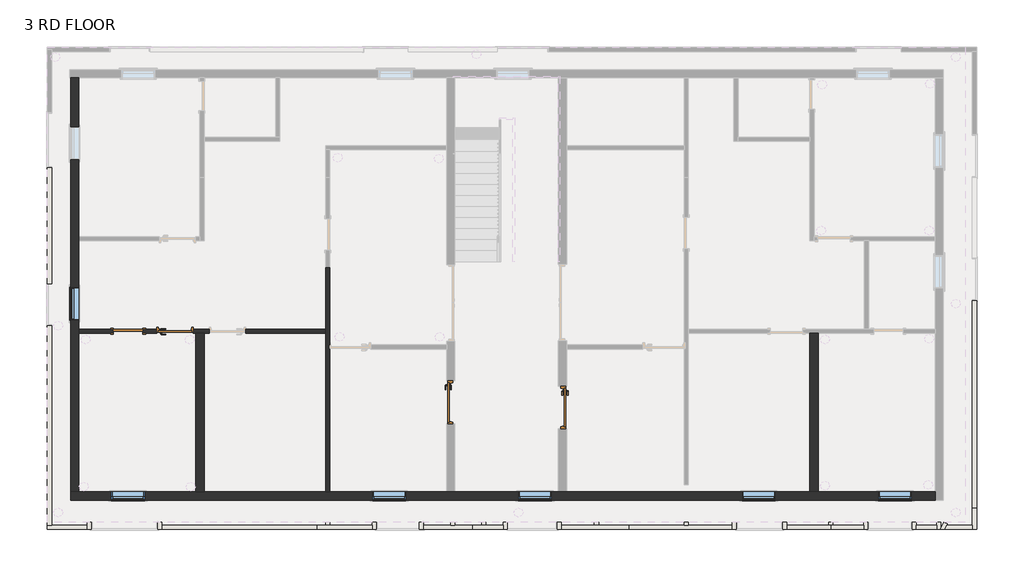
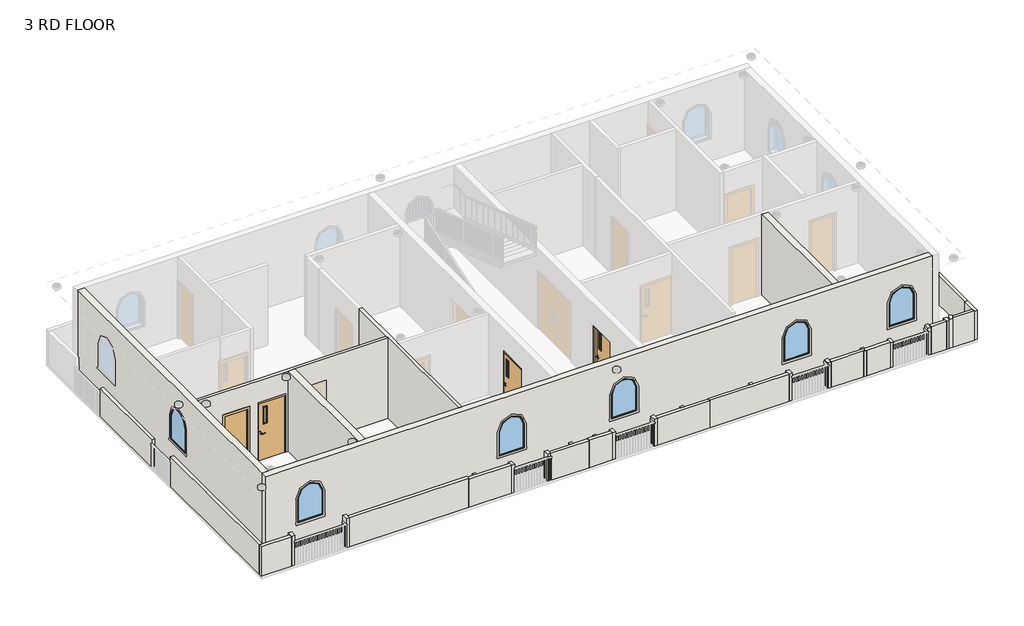
# One storey, part 1 of 7: 39 walls, 6 windows, 4 doors.
# Revit data of these elements (continued)
# Element 4 (IfcDoor, "Single-Flush : 2'8\"x 7'") (continued)
#   Phase Created = New Construction
#   Materials on its faces: "Door - Frame", "Door - Panel"
# Elements 5, 6 (IfcWall, "Generic - 4.5\"")
#   Top Offset = -0' - 6"
#   Base Offset = 0' - 0"
#   wall height = 10' - 0"
#   Phase Created = New Construction
#   Base Constraint = 3 RD FLOOR
#   Top Constraint = 4 TH FLOOR
#   Materials on its faces: "Default Wall"
# Element 7 (IfcWall, "Generic - 4.5\"")
#   Top Offset = -6' - 10.1834"
#   Base Offset = 0' - 0"
#   wall height = 3' - 7.8166"
#   Phase Created = New Construction
#   Base Constraint = 3 RD FLOOR
#   Top Constraint = 4 TH FLOOR
#   Materials on its faces: "Default Wall"
# Element 8 (IfcWall, "Generic - 4.5\"")
#   Top Offset = 0' - 0"
#   Base Offset = 0' - 0"
#   Unconnected Height = 3' - 8.64293"
#   wall height = 3' - 8.64293"
#   Phase Created = New Construction
#   Base Constraint = 3 RD FLOOR
#   Materials on its faces: "Default Wall"
# Element 9 (IfcWall, "Generic - 4.5\"")
#   Top Offset = -6' - 10.57009"
#   Base Offset = 0' - 0"
#   wall height = 3' - 7.42991"
#   Phase Created = New Construction
#   Base Constraint = 3 RD FLOOR
#   Top Constraint = 4 TH FLOOR
#   Materials on its faces: "Default Wall"
# Element 10 (IfcWall, "Generic - 4.5\"")
#   Top Offset = -6' - 11.10495"
#   Base Offset = 0' - 0"
#   wall height = 3' - 6.89505"
#   Phase Created = New Construction
#   Base Constraint = 3 RD FLOOR
#   Top Constraint = 4 TH FLOOR
#   Materials on its faces: "Default Wall"
# Element 11 (IfcWall, "Generic - 4.5\"")
#   Top Offset = -6' - 11.01332"
#   Base Offset = 0' - 0"
#   wall height = 3' - 6.98668"
#   Phase Created = New Construction
#   Base Constraint = 3 RD FLOOR
#   Top Constraint = 4 TH FLOOR
#   Materials on its faces: "Default Wall"
# Element 12 (IfcWall, "Generic - 4.5\"")
#   Top Offset = -7' - 0.14651"
#   Base Offset = 0' - 0"
#   wall height = 3' - 5.85349"
#   Phase Created = New Construction
#   Base Constraint = 3 RD FLOOR
#   Top Constraint = 4 TH FLOOR
#   Materials on its faces: "Default Wall"
# Element 13 (IfcWall, "Generic - 4.5\"")
#   Top Offset = -6' - 11.98199"
#   Base Offset = 0' - 0"
#   wall height = 3' - 6.01801"
#   Phase Created = New Construction
#   Base Constraint = 3 RD FLOOR
#   Top Constraint = 4 TH FLOOR
#   Materials on its faces: "Default Wall"
# Elements 14, 16 (IfcWall, "Generic - 4.5\"")
#   Top Offset = -7' - 2"
#   Base Offset = 0' - 0"
#   wall height = 3' - 4"
#   Phase Created = New Construction
#   Base Constraint = 3 RD FLOOR
#   Top Constraint = 4 TH FLOOR
#   Materials on its faces: "Default Wall"
# Element 15 (IfcWall, "Generic - 4.5\"")
#   Top Offset = -7' - 1.47546"
#   Base Offset = 0' - 0"
#   wall height = 3' - 4.52454"
#   Phase Created = New Construction
#   Base Constraint = 3 RD FLOOR
#   Top Constraint = 4 TH FLOOR
#   Materials on its faces: "Default Wall"
# Elements 17, 33, 34 (IfcWall, "Generic - 4.5\"")
#   Top Offset = -7' - 2.10925"
#   Base Offset = 0' - 0"
#   wall height = 3' - 3.89075"
#   Phase Created = New Construction
#   Base Constraint = 3 RD FLOOR
#   Top Constraint = 4 TH FLOOR
#   Materials on its faces: "Default Wall"
# Elements 18, 19 (IfcWall, "Generic - 4.5\"")
#   Top Offset = -7' - 1.54885"
#   Base Offset = 0' - 0"
#   wall height = 3' - 4.45115"
#   Phase Created = New Construction
#   Base Constraint = 3 RD FLOOR
#   Top Constraint = 4 TH FLOOR
#   Materials on its faces: "Default Wall"
# Element 20 (IfcWall, "Generic - 4.5\"")
#   Top Offset = -7' - 1.35503"
#   Base Offset = 0' - 0"
#   wall height = 3' - 4.64497"
#   Phase Created = New Construction
#   Base Constraint = 3 RD FLOOR
#   Top Constraint = 4 TH FLOOR
#   Materials on its faces: "Default Wall"
# Element 21 (IfcWall, "Generic - 4.5\"")
#   Top Offset = -7' - 3.70017"
#   Base Offset = 0' - 0"
#   wall height = 3' - 2.29983"
#   Phase Created = New Construction
#   Base Constraint = 3 RD FLOOR
#   Top Constraint = 4 TH FLOOR
#   Materials on its faces: "Default Wall"
# Element 22 (IfcWall, "Generic - 4.5\"")
#   Top Offset = -7' - 3.69456"
#   Base Offset = 0' - 0"
#   wall height = 3' - 2.30544"
#   Phase Created = New Construction
#   Base Constraint = 3 RD FLOOR
#   Top Constraint = 4 TH FLOOR
#   Materials on its faces: "Default Wall"
# Element 23 (IfcWall, "Generic - 4.5\"")
#   Top Offset = -7' - 4.34583"
#   Base Offset = 0' - 0"
#   wall height = 3' - 1.65417"
#   Phase Created = New Construction
#   Base Constraint = 3 RD FLOOR
#   Top Constraint = 4 TH FLOOR
#   Materials on its faces: "Default Wall"
# Element 24 (IfcWall, "Generic - 4.5\"")
#   Top Offset = -7' - 3.82361"
#   Base Offset = 0' - 0"
#   wall height = 3' - 2.17639"
#   Phase Created = New Construction
#   Base Constraint = 3 RD FLOOR
#   Top Constraint = 4 TH FLOOR
#   Materials on its faces: "Default Wall"
# Element 25 (IfcWall, "Generic - 4.5\"")
#   Top Offset = -7' - 4.51157"
#   Base Offset = 0' - 0"
#   wall height = 3' - 1.48843"
#   Phase Created = New Construction
#   Base Constraint = 3 RD FLOOR
#   Top Constraint = 4 TH FLOOR
#   Materials on its faces: "Default Wall"
# Element 26 (IfcWall, "Generic - 4.5\"")
#   Top Offset = -7' - 1.5942"
#   Base Offset = 0' - 0"
#   wall height = 3' - 4.4058"
#   Phase Created = New Construction
#   Base Constraint = 3 RD FLOOR
#   Top Constraint = 4 TH FLOOR
#   Materials on its faces: "Default Wall"
# Elements 27, 28 (IfcWall, "Generic - 4.5\"")
#   Top Offset = -7' - 0.71294"
#   Base Offset = 0' - 0"
#   wall height = 3' - 5.28706"
#   Phase Created = New Construction
#   Base Constraint = 3 RD FLOOR
#   Top Constraint = 4 TH FLOOR
#   Materials on its faces: "Default Wall"
# Element 29 (IfcWall, "Generic - 4.5\"")
#   Top Offset = -7' - 0.30229"
#   Base Offset = 0' - 0"
#   wall height = 3' - 5.69771"
#   Phase Created = New Construction
#   Base Constraint = 3 RD FLOOR
#   Top Constraint = 4 TH FLOOR
#   Materials on its faces: "Default Wall"
# Element 30 (IfcWall, "Generic - 4.5\"")
#   Top Offset = -7' - 1.97028"
#   Base Offset = 0' - 0"
#   wall height = 3' - 4.02972"
#   Phase Created = New Construction
#   Base Constraint = 3 RD FLOOR
#   Top Constraint = 4 TH FLOOR
#   Materials on its faces: "Default Wall"
# Element 31 (IfcWall, "Generic - 4.5\"")
#   Top Offset = -7' - 1.40393"
#   Base Offset = 0' - 0"
#   wall height = 3' - 4.59607"
#   Phase Created = New Construction
#   Base Constraint = 3 RD FLOOR
#   Top Constraint = 4 TH FLOOR
#   Materials on its faces: "Default Wall"
# Element 32 (IfcWall, "Generic - 4.5\"")
#   Top Offset = -7' - 1.68978"
#   Base Offset = 0' - 0"
#   wall height = 3' - 4.31022"
#   Phase Created = New Construction
#   Base Constraint = 3 RD FLOOR
#   Top Constraint = 4 TH FLOOR
#   Materials on its faces: "Default Wall"
# Elements 35, 36 (IfcWall, "Generic - 4.5\"")
#   Top Offset = -6' - 10.38959"
#   Base Offset = 0' - 0"
#   wall height = 3' - 7.61041"
#   Phase Created = New Construction
#   Base Constraint = 3 RD FLOOR
#   Top Constraint = 4 TH FLOOR
#   Materials on its faces: "Default Wall"
# Element 37 (IfcWall, "Generic - 4.5\"")
#   Top Offset = 0' - 0"
#   Base Offset = 0' - 0"
#   Unconnected Height = 3' - 7.86488"
#   wall height = 3' - 7.86488"
#   Phase Created = New Construction
#   Base Constraint = 3 RD FLOOR
#   Materials on its faces: "Default Wall"
# Element 38 (IfcWall, "Generic - 4.5\"")
#   Top Offset = -7' - 0.76215"
#   Base Offset = 0' - 0"
#   wall height = 3' - 5.23785"
#   Phase Created = New Construction
#   Base Constraint = 3 RD FLOOR
#   Top Constraint = 4 TH FLOOR
#   Materials on its faces: "Default Wall"
# Element 39 (IfcWall, "Generic - 4.5\"")
#   Top Offset = -6' - 11.21767"
#   Base Offset = 0' - 0"
#   wall height = 3' - 6.78233"
#   Phase Created = New Construction
#   Base Constraint = 3 RD FLOOR
#   Top Constraint = 4 TH FLOOR
#   Materials on its faces: "Default Wall"
# Elements 40, 41, 42, 43 (IfcWall, "Generic - 9\"")
#   Top Offset = -0' - 6"
#   Base Offset = 0' - 0"
#   wall height = 10' - 0"
#   Phase Created = New Construction
#   Base Constraint = 3 RD FLOOR
#   Top Constraint = 4 TH FLOOR
#   Materials on its faces: "Concrete Masonry Units"
# Element 44 (IfcWindow, "Window-Fixed-Round-Top : 3' x 4'")
#   Mark = "145"
#   Window Inset = 0' - 0"
#   Interior Wall Closure = 0' - 2 1/4"
#   Frame Extension = 0' - 0 1/4"
#   Exterior Wall Closure = 0' - 1 1/4"
#   Interior Trim Visibility = yes
#   Exterior Trim Visibility = yes
#   Phase Created = New Construction
#   Materials on its faces: "Wood - Stained", "Clad - White", "Glass"
# Element 45 (IfcWindow, "Window-Fixed-Round-Top : 3' x 4'")
#   Mark = "146"
#   Window Inset = 0' - 0"
#   Interior Wall Closure = 0' - 2 1/4"
#   Frame Extension = 0' - 0 1/4"
#   Exterior Wall Closure = 0' - 1 1/4"
#   Interior Trim Visibility = yes
#   Exterior Trim Visibility = yes
#   Phase Created = New Construction
#   Materials on its faces: "Wood - Stained", "Clad - White", "Glass"
# Element 46 (IfcWindow, "Window-Fixed-Round-Top : 3' x 4'")
#   Mark = "147"
#   Window Inset = 0' - 0"
#   Interior Wall Closure = 0' - 2 1/4"
#   Frame Extension = 0' - 0 1/4"
#   Exterior Wall Closure = 0' - 1 1/4"
#   Interior Trim Visibility = yes
#   Exterior Trim Visibility = yes
#   Phase Created = New Construction
#   Materials on its faces: "Wood - Stained", "Clad - White", "Glass"
# Element 47 (IfcWindow, "Window-Fixed-Round-Top : 3' x 4'")
#   Mark = "148"
#   Window Inset = 0' - 0"
#   Interior Wall Closure = 0' - 2 1/4"
#   Frame Extension = 0' - 0 1/4"
#   Exterior Wall Closure = 0' - 1 1/4"
#   Interior Trim Visibility = yes
#   Exterior Trim Visibility = yes
#   Phase Created = New Construction
#   Materials on its faces: "Wood - Stained", "Clad - White", "Glass"
# Element 48 (IfcWindow, "Window-Fixed-Round-Top : 3' x 4'")
#   Mark = "149"
#   Window Inset = 0' - 0"
#   Interior Wall Closure = 0' - 2 1/4"
#   Frame Extension = 0' - 0 1/4"
#   Exterior Wall Closure = 0' - 1 1/4"
#   Interior Trim Visibility = yes
#   Exterior Trim Visibility = yes
#   Phase Created = New Construction
#   Materials on its faces: "Wood - Stained", "Clad - White", "Glass"
# Element 49 (IfcWindow, "Window-Fixed-Round-Top : 3' x 4'")
#   Mark = "157"
#   Window Inset = 0' - 0"
#   Interior Wall Closure = 0' - 2 1/4"
#   Frame Extension = 0' - 0 1/4"
#   Exterior Wall Closure = 0' - 1 1/4"
#   Interior Trim Visibility = yes
#   Exterior Trim Visibility = yes
#   Phase Created = New Construction
#   Materials on its faces: "Wood - Stained", "Clad - White", "Glass"
# Materials
#   "Wood - Birch": class "Wood", colour RGB 166 116 52, transparency 0, Cost = 0
#   "Glass": class "Glass", colour RGB 0 128 192, transparency 0.75, Description = "Soda Lime Glass", Cost = 0
#   "Metal - Paint Finish - Grey": class "Paint", colour RGB 104 104 104, transparency 0, Cost = 0
#   "Aluminum": class "Metal", colour RGB 247 247 247, transparency 0, Description = "Aluminum 6061", Cost = 0
#   "Door - Panel": class "Wood", colour RGB 210 159 95, transparency 0, Cost = 0
#   "Door - Frame": colour RGB 118 70 51, transparency 0, Cost = 0
#   "Concrete Masonry Units": class "Masonry", colour RGB 227 227 227, transparency 0, Description = "Concrete masonry units", Cost = 0
#   "Wood - Stained": class "Wood", colour RGB 224 178 126, transparency 0, Cost = 0
#   "Clad - White": class "Wood", colour RGB 242 242 238, transparency 0, Cost = 0
#   "Default Wall": colour RGB 128 128 128, transparency 0, Cost = 0
